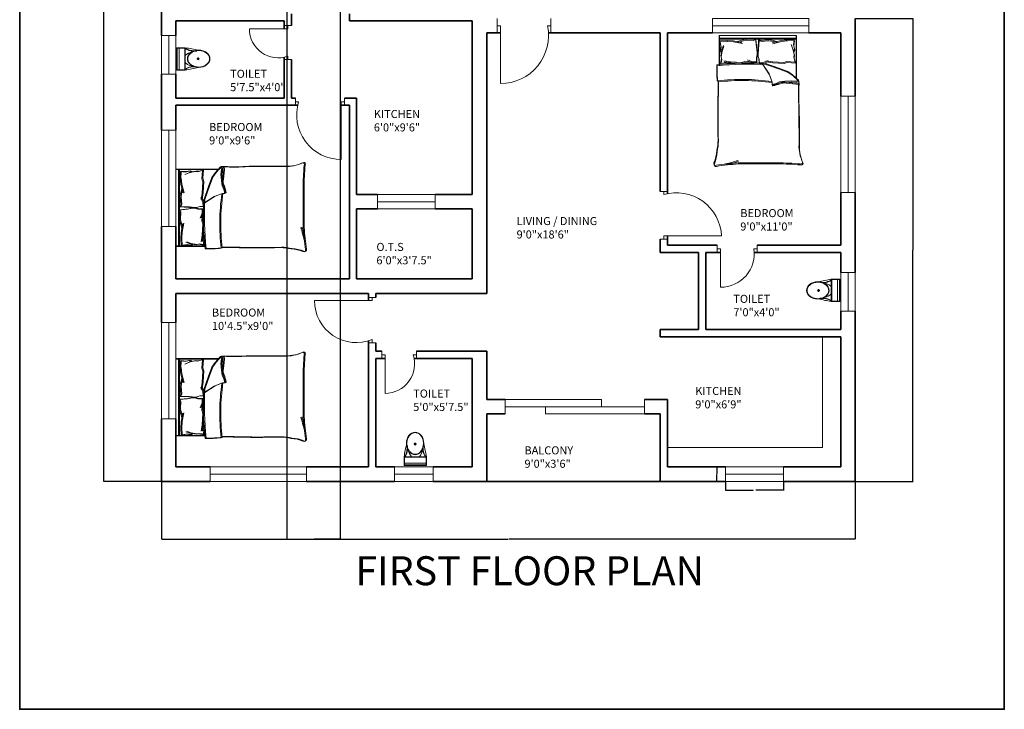
# Model space of a CAD drawing. Units: inches. Extents: x 2527 to 3140, y 1564 to 2435.
# Tile 1 of 4: x 2527 to 3140, y 1564 to 1993. Entities that reach past the tile are written whole.
import ezdxf

# ---------------------------------------------------------------- set-up
doc = ezdxf.new("R2010")
doc.units = ezdxf.units.IN
for name, color, linetype, lineweight in [('A-ANNO-DIMS', 2, 'Continuous', 18), ('A-ANNO-TEXT', 7, 'Continuous', 25), ('A-ANNO-TTLB', 7, 'Continuous', 35), ('A-AREA-IDEN', 7, 'Continuous', 18), ('A-DOOR', 191, 'Continuous', 18), ('A-FLOR-CASE', 9, 'Continuous', 18), ('A-FLOR-FIXT', 7, 'Continuous', 18), ('A-FURN', 8, 'Continuous', 13), ('A-GLAZ', 131, 'Continuous', 18), ('A-WALL', 7, 'Continuous', 35)]:
    doc.layers.add(name, color=color, linetype=linetype, lineweight=lineweight)
doc.styles.get("Standard").update_dxf_attribs({"font": 'arial.ttf'})
doc.dimstyles.get("Standard").update_dxf_attribs({"dimtxt": 0.18, "dimasz": 0.18, "dimexe": 0.18, "dimexo": 0.0625, "dimgap": 0.09, "dimtad": 0, "dimtih": 1, "dimtoh": 1, "dimdec": 4, "dimzin": 0, "dimdsep": 46, "dimtxsty": 'Standard', "dimcen": 0.09, "dimadec": 0, "dimazin": 0, "dimtfac": 1, "dimtdec": 4, "dimtofl": 0, "dimtmove": 0, "dimatfit": 3, "dimfxl": 1, "dimtolj": 1, "dimtzin": 0, "dimarcsym": 0})

# ---------------------------------------------------------------- blocks, each defined once
blk = doc.blocks.new('A$C31115884')
for p, q in [((283, 498), (223, 498)), ((258, 466), (258, 523)), ((0, 200), (0, 0)), ((520, 200), (0, 200)), ((510, 54), (0, 54)), ((10, 190), (10, 10)), ((510, 190), (10, 190)), ((10, 10), (510, 10)), ((510, 10), (510, 190)), ((520, 0), (520, 200)), ((0, 0), (520, 0))]:
    blk.add_line(p, q)
blk.add_circle((256, 496), 23.6)
for centre, radius, start, end in [((2778, -205), 2807, 165.4549, 171.7133), ((-295, 403), 365, 324.2091, 9.3499), ((-295, 403), 375, 324.2091, 9.3499), ((806, 403), 365, 170.6501, 215.7909), ((3237, 905), 2807, 188.2867, 194.5451), ((384, 406), 293, 190.2774, 224.1564), ((139, 406), 293, 315.8436, 2.6563), ((806, 403), 375, 179.2036, 215.7909)]:
    blk.add_arc(centre, radius, start, end)
blk.add_ellipse((256, 510), major_axis=(0, -261), ratio=0.772727)
blk.add_open_spline([(256, 259), (263, 259), (270, 260), (288, 262), (299, 265), (320, 273), (330, 278), (350, 291), (360, 299), (378, 316), (386, 326), (402, 347), (409, 358), (421, 383), (427, 395), (436, 422), (440, 436), (445, 465), (447, 480), (448, 509), (448, 524), (445, 553), (443, 568), (436, 596), (432, 610), (422, 636), (416, 649), (402, 672), (395, 683), (379, 703), (370, 712), (351, 728), (341, 735), (321, 746), (310, 751), (289, 757), (278, 759), (256, 761), (245, 761), (223, 757), (212, 754), (191, 746), (181, 741), (161, 728), (151, 720), (133, 703), (125, 693), (110, 672), (103, 660), (90, 636), (85, 623), (76, 596), (72, 582), (67, 553), (66, 538), (64, 509), (65, 494), (68, 465), (70, 450), (77, 422), (81, 408), (91, 382), (97, 370), (111, 346), (118, 335), (135, 316), (144, 307), (162, 291), (172, 284), (193, 273), (203, 269), (225, 262), (236, 260), (250, 259), (253, 259), (256, 259)], degree=3, knots=[0, 0, 0, 0, 0.110105, 0.110105, 0.285049, 0.285049, 0.459994, 0.459994, 0.634938, 0.634938, 0.809882, 0.809882, 0.984827, 0.984827, 1.159771, 1.159771, 1.334715, 1.334715, 1.50966, 1.50966, 1.684604, 1.684604, 1.859549, 1.859549, 2.034493, 2.034493, 2.209437, 2.209437, 2.384382, 2.384382, 2.559326, 2.559326, 2.73427, 2.73427, 2.909215, 2.909215, 3.084159, 3.084159, 3.259103, 3.259103, 3.434048, 3.434048, 3.608992, 3.608992, 3.783936, 3.783936, 3.958881, 3.958881, 4.133825, 4.133825, 4.30877, 4.30877, 4.483714, 4.483714, 4.658658, 4.658658, 4.833603, 4.833603, 5.008547, 5.008547, 5.183491, 5.183491, 5.358436, 5.358436, 5.53338, 5.53338, 5.708324, 5.708324, 5.883269, 5.883269, 6.058213, 6.058213, 6.233158, 6.233158, 6.283185, 6.283185, 6.283185, 6.283185])
blk = doc.blocks.new('BED-DOUBLE')
for p, q in [((3.48, 63.33), (3.48, 81.44)), ((3.48, 63.33), (3.48, 81.44)), ((3.48, 81.44), (51.49, 81.44)), ((3.48, 79.91), (51.27, 79.91)), ((3.48, 79.91), (51.27, 79.91)), ((3.7, 62.69), (3.7, 80.8)), ((3.7, 62.69), (3.7, 80.8)), ((51.27, 81.44), (51.27, 54.83)), ((51.27, 81.44), (51.27, 54.83)), ((51.49, 81.44), (51.49, 80.8)), ((51.49, 80.8), (51.49, 54.19)), ((51.49, 80.8), (51.49, 54.19)), ((3.7, 79.27), (51.49, 79.27)), ((3.7, 79.27), (51.49, 79.27)), ((3.89, 78.13), (4.47, 74.95)), ((3.9, 78.1), (8.18, 78.43)), ((3.9, 78.1), (8.18, 78.43)), ((3.9, 78.13), (4.47, 74.95)), ((4.47, 74.95), (4.04, 72.34)), ((4.47, 74.95), (4.04, 72.34)), ((4.12, 77.49), (4.7, 74.31)), ((4.12, 77.49), (4.7, 74.31)), ((4.13, 77.47), (8.41, 77.79)), ((4.13, 77.47), (8.41, 77.79)), ((4.7, 74.31), (4.27, 71.7)), ((4.7, 74.31), (4.27, 71.7)), ((5.05, 72.49), (6.06, 75.24)), ((5.05, 72.49), (6.06, 75.24)), ((5.28, 71.85), (6.29, 74.6)), ((5.28, 71.85), (6.29, 74.6)), ((8.18, 78.43), (8.29, 78.42)), ((8.18, 78.43), (8.29, 78.42)), ((8.29, 78.42), (12.11, 78.13)), ((8.29, 78.42), (12.11, 78.13)), ((8.41, 77.79), (8.51, 77.78)), ((8.41, 77.79), (8.51, 77.78)), ((8.51, 77.78), (12.34, 77.49)), ((8.51, 77.78), (12.34, 77.49)), ((12.11, 78.13), (17.6, 77.11)), ((12.11, 78.13), (17.6, 77.11)), ((12.34, 77.49), (17.83, 76.48)), ((12.34, 77.49), (17.83, 76.48)), ((14.86, 77.69), (16.88, 78.42)), ((14.86, 77.69), (16.88, 78.42)), ((15.08, 77.05), (17.11, 77.78)), ((15.08, 77.05), (17.11, 77.78)), ((16.88, 78.42), (19.77, 79.14)), ((16.88, 78.42), (19.77, 79.14)), ((17.11, 77.78), (20, 78.5)), ((17.11, 77.78), (20, 78.5)), ((19.77, 79.14), (20.09, 79.14)), ((19.77, 79.14), (20.09, 79.14)), ((20, 78.5), (20.32, 78.5)), ((20, 78.5), (20.32, 78.5)), ((20.09, 79.14), (24.54, 78.99)), ((20.09, 79.14), (24.54, 78.99)), ((20.32, 78.5), (24.77, 78.35)), ((20.32, 78.5), (24.77, 78.35)), ((24.54, 78.99), (25.98, 79.57)), ((24.54, 78.99), (25.98, 79.57)), ((24.77, 78.35), (26.21, 78.93)), ((24.77, 78.35), (26.21, 78.93)), ((25.98, 79.57), (26.56, 74.22)), ((25.98, 79.57), (26.56, 74.22)), ((26.21, 78.93), (26.79, 73.58)), ((26.21, 78.93), (26.79, 73.58)), ((26.56, 74.22), (27.14, 71.04)), ((26.56, 74.22), (27.14, 71.04)), ((26.79, 73.58), (27.37, 70.4)), ((26.79, 73.58), (27.37, 70.4)), ((27.73, 73.58), (27.36, 70.36)), ((27.73, 73.58), (27.36, 70.36)), ((27.98, 78.95), (27.73, 73.58)), ((27.98, 78.95), (27.73, 73.58)), ((28.21, 78.31), (27.96, 72.94)), ((28.21, 78.31), (27.96, 72.94)), ((29.46, 78.46), (27.98, 78.95)), ((29.46, 78.46), (27.98, 78.95)), ((29.68, 77.82), (28.21, 78.31)), ((29.68, 77.82), (28.21, 78.31)), ((33.88, 78.89), (29.46, 78.46)), ((33.88, 78.89), (29.46, 78.46)), ((34.11, 78.25), (29.68, 77.82)), ((34.11, 78.25), (29.68, 77.82)), ((34.21, 78.91), (33.88, 78.89)), ((34.2, 78.91), (33.88, 78.89)), ((34.43, 78.27), (34.11, 78.25)), ((34.43, 78.27), (34.11, 78.25)), ((37.14, 78.36), (34.2, 78.91)), ((37.14, 78.36), (34.21, 78.91)), ((37.36, 77.73), (34.43, 78.27)), ((37.36, 77.73), (34.43, 78.27)), ((41.91, 78.37), (36.5, 77.02)), ((41.91, 78.37), (36.5, 77.02)), ((42.14, 77.73), (36.72, 76.38)), ((42.14, 77.73), (36.72, 76.38)), ((39.2, 77.77), (37.14, 78.36)), ((39.2, 77.77), (37.14, 78.36)), ((39.43, 77.13), (37.36, 77.73)), ((39.43, 77.13), (37.36, 77.73)), ((45.71, 78.9), (41.91, 78.37)), ((45.71, 78.9), (41.91, 78.37)), ((45.94, 78.26), (42.14, 77.73)), ((45.94, 78.26), (42.14, 77.73)), ((50.11, 78.89), (44.71, 78.98)), ((44.71, 78.98), (45.71, 78.9)), ((50.11, 78.89), (44.71, 78.98)), ((44.71, 78.98), (45.71, 78.9)), ((50.34, 78.25), (44.94, 78.34)), ((44.94, 78.34), (45.94, 78.26)), ((50.34, 78.25), (44.94, 78.34)), ((44.94, 78.34), (45.94, 78.26)), ((49.31, 73.19), (48.13, 75.86)), ((49.31, 73.19), (48.13, 75.86)), ((49.54, 72.55), (48.36, 75.23)), ((49.54, 72.55), (48.36, 75.23)), ((50.11, 78.89), (49.73, 75.68)), ((50.11, 78.89), (49.73, 75.68)), ((49.73, 75.68), (50.33, 73.1)), ((49.73, 75.68), (50.33, 73.1)), ((50.34, 78.25), (49.96, 75.04)), ((50.34, 78.25), (49.96, 75.04)), ((49.96, 75.04), (50.56, 72.47)), ((49.96, 75.04), (50.56, 72.47)), ((4.04, 72.34), (4.62, 71.33)), ((4.04, 72.34), (4.62, 71.33)), ((4.27, 71.7), (4.85, 70.69)), ((4.27, 71.7), (4.85, 70.69)), ((4.47, 68.87), (5.05, 72.49)), ((4.47, 68.87), (5.05, 72.49)), ((4.76, 67.28), (4.47, 68.87)), ((4.76, 67.28), (4.47, 68.87)), ((4.7, 68.23), (5.28, 71.85)), ((4.7, 68.23), (5.28, 71.85)), ((4.99, 66.64), (4.7, 68.23)), ((4.99, 66.64), (4.7, 68.23)), ((27.14, 69.74), (26.56, 67.86)), ((27.14, 69.74), (26.56, 67.86)), ((26.56, 67.86), (26.56, 65.18)), ((26.56, 67.86), (26.56, 65.18)), ((27.37, 69.1), (26.79, 67.22)), ((27.37, 69.1), (26.79, 67.22)), ((27.14, 71.04), (27.14, 69.74)), ((27.14, 71.04), (27.14, 69.74)), ((27.36, 70.36), (27.44, 69.07)), ((27.36, 70.36), (27.44, 69.07)), ((27.37, 70.4), (27.37, 69.1)), ((27.37, 70.4), (27.37, 69.1)), ((27.44, 69.07), (28.13, 67.23)), ((27.44, 69.07), (28.13, 67.23)), ((27.96, 72.94), (27.58, 69.73)), ((27.96, 72.94), (27.58, 69.73)), ((27.58, 69.73), (27.66, 68.43)), ((27.58, 69.73), (27.66, 68.43)), ((27.66, 68.43), (28.36, 66.59)), ((27.66, 68.43), (28.36, 66.59)), ((50.11, 69.61), (49.31, 73.19)), ((50.11, 69.61), (49.31, 73.19)), ((50.34, 68.97), (49.54, 72.55)), ((50.34, 68.97), (49.54, 72.55)), ((50.33, 73.1), (49.81, 72.06)), ((50.33, 73.1), (49.82, 72.06)), ((49.92, 68.01), (50.11, 69.61)), ((49.92, 68.01), (50.11, 69.61)), ((50.7, 64.87), (49.92, 68.01)), ((50.7, 64.87), (49.92, 68.01)), ((50.56, 72.47), (50.04, 71.42)), ((50.56, 72.47), (50.04, 71.42)), ((50.15, 67.37), (50.34, 68.97)), ((50.15, 67.37), (50.34, 68.97)), ((4.18, 64.1), (4.76, 67.28)), ((4.18, 64.1), (4.76, 67.28)), ((9.28, 64.82), (4.18, 64.1)), ((9.28, 64.82), (4.18, 64.1)), ((4.41, 63.46), (4.99, 66.64)), ((4.41, 63.46), (4.99, 66.64)), ((9.51, 64.19), (4.41, 63.46)), ((9.51, 64.19), (4.41, 63.46)), ((6.38, 65.81), (10.41, 65.15)), ((6.38, 65.81), (10.41, 65.15)), ((6.61, 65.17), (10.64, 64.51)), ((6.61, 65.17), (10.64, 64.51)), ((10.41, 65.15), (9.28, 64.82)), ((10.41, 65.15), (9.28, 64.82)), ((10.64, 64.51), (9.51, 64.19)), ((10.64, 64.51), (9.51, 64.19)), ((10.41, 65.15), (17.42, 64.72)), ((10.41, 65.15), (17.42, 64.72)), ((10.64, 64.51), (17.65, 64.08)), ((10.64, 64.51), (17.65, 64.08)), ((17.42, 64.72), (19.38, 65.27)), ((17.42, 64.72), (19.38, 65.27)), ((17.65, 64.08), (19.61, 64.63)), ((17.65, 64.08), (19.61, 64.63)), ((19.38, 65.27), (24.52, 64.87)), ((19.38, 65.27), (24.52, 64.87)), ((19.61, 64.63), (24.74, 64.23)), ((19.61, 64.63), (24.74, 64.23)), ((24.1, 65.18), (20.96, 66.27)), ((24.1, 65.18), (20.96, 66.27)), ((24.33, 64.54), (21.19, 65.63)), ((24.33, 64.54), (21.19, 65.63)), ((26.56, 65.18), (24.1, 65.18)), ((26.56, 65.18), (24.1, 65.18)), ((26.79, 64.54), (24.33, 64.54)), ((26.79, 64.54), (24.33, 64.54)), ((26.79, 67.22), (26.79, 64.54)), ((26.79, 67.22), (26.79, 64.54)), ((28.13, 67.23), (28.3, 64.55)), ((28.13, 67.23), (28.3, 64.55)), ((28.3, 64.55), (30.75, 64.7)), ((28.3, 64.55), (30.75, 64.7)), ((28.36, 66.59), (28.53, 63.91)), ((28.36, 66.59), (28.53, 63.91)), ((28.53, 63.91), (30.98, 64.06)), ((28.53, 63.91), (30.98, 64.06)), ((30.26, 64.06), (34.45, 57.57)), ((30.26, 64.06), (34.45, 57.57)), ((30.49, 63.42), (34.68, 56.93)), ((30.49, 63.42), (34.68, 56.93)), ((30.75, 64.7), (33.82, 65.99)), ((30.75, 64.7), (33.82, 65.99)), ((30.98, 64.06), (34.05, 65.35)), ((30.98, 64.06), (34.05, 65.35)), ((40.64, 61.13), (32.31, 64.06)), ((40.64, 61.13), (32.31, 64.06)), ((40.87, 60.49), (32.53, 63.42)), ((40.87, 60.49), (32.54, 63.42)), ((32.56, 65.81), (36.6, 65.15)), ((32.56, 65.81), (36.6, 65.15)), ((32.79, 65.17), (36.83, 64.51)), ((32.79, 65.17), (36.82, 64.51)), ((36.6, 65.15), (43.61, 64.72)), ((36.6, 65.15), (43.61, 64.72)), ((36.82, 64.51), (43.83, 64.08)), ((36.83, 64.51), (43.84, 64.08)), ((43.61, 64.72), (45.57, 65.27)), ((43.61, 64.72), (45.57, 65.27)), ((43.83, 64.08), (45.8, 64.63)), ((43.84, 64.08), (45.8, 64.63)), ((45.57, 65.27), (50.7, 64.87)), ((45.57, 65.27), (50.7, 64.87)), ((45.8, 64.63), (50.93, 64.23)), ((45.8, 64.63), (50.93, 64.23)), ((50.93, 64.23), (50.15, 67.37)), ((50.93, 64.23), (50.15, 67.37)), ((34.45, 57.57), (36.15, 53.08)), ((34.45, 57.57), (36.15, 53.08)), ((34.68, 56.93), (36.38, 52.44)), ((34.68, 56.93), (36.38, 52.44)), ((46.22, 59.11), (40.64, 61.13)), ((46.22, 59.11), (40.64, 61.13)), ((46.45, 58.47), (40.87, 60.49)), ((46.45, 58.47), (40.87, 60.49)), ((49.16, 56.95), (46.22, 59.11)), ((49.16, 56.95), (46.22, 59.11)), ((49.39, 56.31), (46.45, 58.47)), ((49.39, 56.31), (46.45, 58.47)), ((52.87, 53.7), (49.16, 56.95)), ((52.87, 53.7), (49.16, 56.95)), ((53.1, 53.06), (49.39, 56.31)), ((53.1, 53.06), (49.39, 56.31)), ((36.15, 53.08), (36.46, 51.07)), ((36.15, 53.08), (36.46, 51.07)), ((36.38, 52.44), (36.69, 50.43)), ((36.38, 52.44), (36.69, 50.43)), ((36.46, 51.07), (38.94, 51.68)), ((36.46, 51.07), (38.94, 51.68)), ((36.69, 50.43), (39.17, 51.05)), ((36.69, 50.43), (39.17, 51.05)), ((38.94, 51.68), (40.95, 52.61)), ((38.94, 51.68), (40.95, 52.61)), ((39.17, 51.05), (41.18, 51.97)), ((39.17, 51.05), (41.18, 51.97)), ((40.95, 52.61), (44.36, 53.08)), ((40.95, 52.61), (44.36, 53.08)), ((41.18, 51.97), (44.59, 52.44)), ((41.18, 51.97), (44.59, 52.44)), ((44.36, 53.08), (48.23, 53.39)), ((44.36, 53.08), (48.23, 53.39)), ((44.59, 52.44), (48.46, 52.75)), ((44.59, 52.44), (48.46, 52.75)), ((48.23, 53.39), (51.33, 53.08)), ((48.23, 53.39), (51.33, 53.08)), ((48.46, 52.75), (51.56, 52.44)), ((48.46, 52.75), (51.56, 52.44)), ((51.33, 53.08), (52.87, 53.7)), ((51.33, 53.08), (52.87, 53.7)), ((51.56, 52.44), (53.1, 53.06)), ((51.56, 52.44), (53.1, 53.06)), ((52.95, 51.95), (52.87, 53.7, 3.87)), ((52.95, 51.95), (52.87, 53.7, 3.87)), ((53.18, 51.31), (53.1, 53.06, 3.87)), ((53.18, 51.31), (53.1, 53.06, 3.87)), ((15.06, 2.2), (39.68, 2.2)), ((15.06, 2.2), (39.68, 2.2)), ((15.29, 1.56), (39.91, 1.56)), ((15.29, 1.56), (39.91, 1.56))]:
    blk.add_line(p, q)
for centre, radius, start, end in [((85.16, 61.35), 83.31, 178.72178, 185.60397), ((85.16, 61.35), 83.31, 178.72178, 185.60397), ((21.36, -100.61), 164.97, 86.08655, 96.78213), ((21.36, -100.61), 164.97, 86.08655, 96.78213), ((85.39, 60.71), 83.31, 178.72178, 185.60397), ((85.39, 60.71), 83.31, 178.72178, 185.60397), ((21.59, -101.25), 164.97, 86.08655, 96.78213), ((21.59, -101.25), 164.97, 86.08655, 96.78213), ((17.76, -74.87), 129.02, 81.78449, 96.90062), ((17.76, -74.87), 129.02, 81.78449, 96.90062), ((17.98, -75.51), 129.02, 81.78449, 96.90062), ((17.98, -75.51), 129.02, 81.78449, 96.90062), ((-167.31, 50.27), 170.11, 358.4762, 1.00819), ((-167.31, 50.27), 170.11, 358.4762, 1.00819), ((-167.08, 49.63), 170.11, 358.4762, 1.00819), ((-167.08, 49.63), 170.11, 358.4762, 1.00819), ((36.64, 51), 0.185, 160.24637, 271.13765), ((36.64, 51), 0.185, 160.24637, 271.13765), ((31.15, 79.96), 29.65, 280.66171, 289.88058), ((31.15, 79.96), 29.65, 280.66171, 289.88058), ((36.87, 50.36), 0.185, 160.24637, 271.13765), ((36.86, 50.36), 0.185, 160.24637, 271.13765), ((31.38, 79.32), 29.65, 280.66171, 289.88058), ((31.38, 79.32), 29.65, 280.66171, 289.88058), ((43.74, 46.38), 6.22, 78.6608, 113.73842), ((43.74, 46.38), 6.22, 78.6608, 113.73842), ((43.97, 45.74), 6.22, 78.6608, 113.73842), ((43.97, 45.74), 6.22, 78.6608, 113.73842), ((51.33, 88.1), 36.18, 259.87628, 272.56571), ((51.33, 88.1), 36.18, 259.87628, 272.56571), ((51.56, 87.46), 36.18, 259.87628, 272.56571), ((51.56, 87.46), 36.18, 259.87628, 272.56571), ((182.27, 45.13), 129.5, 176.97912, 183.83645), ((182.27, 45.13), 129.5, 176.97912, 183.83645), ((182.49, 44.49), 129.5, 176.97912, 183.83645), ((182.49, 44.49), 129.5, 176.97912, 183.83645), ((484.82, 30.83), 482.31, 178.22771, 181.71854), ((484.82, 30.83), 482.31, 178.22771, 181.71854), ((485.05, 30.19), 482.31, 178.22771, 181.71854), ((485.05, 30.19), 482.31, 178.22771, 181.71854), ((-4508.74, 13.62), 4561.86, 0.00217, 0.28689), ((-4508.74, 13.62), 4561.86, 0.00217, 0.28689), ((-4508.51, 12.98), 4561.86, 0.00217, 0.28689), ((-4508.51, 12.98), 4561.86, 0.00217, 0.28689), ((-26.9, 16.93), 29.63, 346.06484, 358.91125), ((-26.9, 16.93), 29.63, 346.06484, 358.91125), ((-26.67, 16.29), 29.63, 346.06484, 358.91125), ((-26.67, 16.29), 29.63, 346.06484, 358.91125), ((76.16, 12.78), 23.07, 177.47136, 206.46809), ((76.16, 12.78), 23.07, 177.47136, 206.46809), ((76.39, 12.14), 23.07, 177.47136, 206.46809), ((76.39, 12.14), 23.07, 177.47136, 206.46809), ((-21.66, 11.17), 23.56, 337.97508, 356.652), ((-21.66, 11.17), 23.56, 337.97508, 356.652), ((-21.43, 10.53), 23.56, 337.97508, 356.652), ((-21.43, 10.53), 23.56, 337.97508, 356.652), ((1.09, 1.73), 1.09, 146.17358, 293.47814), ((1.09, 1.73), 1.09, 146.17358, 293.47814), ((1.32, 1.09), 1.09, 146.17358, 293.47814), ((1.32, 1.09), 1.09, 146.17358, 293.47814), ((21.43, -119.39), 121.76, 92.99578, 99.40907), ((21.43, -119.39), 121.76, 92.99578, 99.40907), ((21.66, -120.03), 121.76, 92.99578, 99.40907), ((21.66, -120.03), 121.76, 92.99578, 99.40907), ((-17.22, 105.15), 106.46, 283.38322, 287.70533), ((-17.22, 105.15), 106.46, 283.38322, 287.70533), ((-16.99, 104.52), 106.46, 283.38322, 287.70533), ((-16.99, 104.52), 106.46, 283.38322, 287.70533), ((41.15, -130.83), 133.04, 84.4998, 90.63509), ((41.15, -130.83), 133.04, 84.4998, 90.63509), ((41.38, -131.47), 133.04, 84.4998, 90.63509), ((41.38, -131.47), 133.04, 84.4998, 90.63509), ((54.41, 2.57), 1.1, 242.65876, 356.02002), ((54.41, 2.57), 1.1, 242.65876, 356.02002), ((54.64, 1.93), 1.1, 242.65876, 356.02002), ((54.64, 1.93), 1.1, 242.65876, 356.02002)]:
    blk.add_arc(centre, radius, start, end)
blk = doc.blocks.new('WIN-60')
for p, q in [((0, 9), (0, 0)), ((60, 9), (0, 9)), ((60, 4.5), (60, 9)), ((60, 9), (60, 0)), ((0, 0), (0, 4.5)), ((0, 4.5), (60, 4.5)), ((0, 0), (60, 0))]:
    blk.add_line(p, q)
blk = doc.blocks.new('WIN-24')
for p, q in [((4.5, 24), (0, 24)), ((0, 24), (9, 24)), ((0, 24), (0, 0)), ((4.5, 0), (4.5, 24)), ((9, 24), (9, 0)), ((0, 0), (9, 0)), ((9, 0), (4.5, 0))]:
    blk.add_line(p, q)
blk = doc.blocks.new('WIN-36')
for p, q in [((0, 36), (9, 36)), ((0, 36), (0, 0)), ((9, 36), (4.5, 36)), ((4.5, 36), (4.5, 0)), ((9, 36), (9, 0)), ((4.5, 0), (0, 0)), ((0, 0), (9, 0))]:
    blk.add_line(p, q)
blk = doc.blocks.new('*D15')
at = {"layer": 'A-ANNO-DIMS', "color": 0, "lineweight": -2, "transparency": 16777216}
for p, q in [((2966.88, 1706.08), (2966.88, 1700.56)), ((3002.88, 1706.08), (3002.88, 1700.56)), ((2967.06, 1700.74), (2984.03, 1700.74)), ((3002.7, 1700.74), (2985.72, 1700.74))]:
    blk.add_line(p, q, dxfattribs=at)
at = {"layer": 'A-ANNO-DIMS', "color": 0, "transparency": 16777216}
for points in [[(2967.06, 1700.77), (2967.06, 1700.71), (2966.88, 1700.74)], [(3002.7, 1700.77), (3002.7, 1700.71), (3002.88, 1700.74)]]:
    blk.add_solid(points, dxfattribs=at)
at = {"layer": 'Defpoints', "color": 0, "transparency": 16777216}
for p in [(2966.88, 1706.14), (3002.88, 1706.14), (2966.88, 1700.74)]:
    blk.add_point(p, dxfattribs=at)
at = {"layer": 'A-ANNO-DIMS', "color": 0, "transparency": 16777216, "insert": (2984.88, 1700.74), "char_height": 0.18, "attachment_point": 5}
blk.add_mtext('\\A1;WIN. 36 TYP.', dxfattribs=at)
blk = doc.blocks.new('*D16')
at = {"layer": 'A-ANNO-DIMS', "color": 0, "lineweight": -2, "transparency": 16777216}
for p, q in [((2966.82, 1715.14), (2961.3, 1715.14)), ((2961.48, 1714.96), (2961.48, 1710.82)), ((2966.82, 1706.14), (2961.3, 1706.14)), ((2961.48, 1706.32), (2961.48, 1710.46))]:
    blk.add_line(p, q, dxfattribs=at)
at = {"layer": 'A-ANNO-DIMS', "color": 0, "transparency": 16777216}
for points in [[(2961.45, 1714.96), (2961.51, 1714.96), (2961.48, 1715.14)], [(2961.45, 1706.32), (2961.51, 1706.32), (2961.48, 1706.14)]]:
    blk.add_solid(points, dxfattribs=at)
at = {"layer": 'Defpoints', "color": 0, "transparency": 16777216}
for p in [(2961.48, 1715.14), (2966.88, 1715.14), (2966.88, 1706.14)]:
    blk.add_point(p, dxfattribs=at)
at = {"layer": 'A-ANNO-DIMS', "color": 0, "transparency": 16777216, "insert": (2961.48, 1710.64), "char_height": 0.18, "attachment_point": 5}
blk.add_mtext('\\A1;9 TYP.', dxfattribs=at)
blk = doc.blocks.new('*D19')
at = {"layer": 'A-ANNO-DIMS', "color": 0, "lineweight": -2, "transparency": 16777216}
for p, q in [((2615.58, 1706.08), (2615.58, 1670.11)), ((3047.58, 1706.08), (3047.58, 1670.11)), ((2615.76, 1670.29), (2831.29, 1670.29)), ((3047.4, 1670.29), (2831.87, 1670.29))]:
    blk.add_line(p, q, dxfattribs=at)
at = {"layer": 'A-ANNO-DIMS', "color": 0, "transparency": 16777216}
for points in [[(2615.76, 1670.32), (2615.76, 1670.26), (2615.58, 1670.29)], [(3047.4, 1670.32), (3047.4, 1670.26), (3047.58, 1670.29)]]:
    blk.add_solid(points, dxfattribs=at)
at = {"layer": 'Defpoints', "color": 0, "transparency": 16777216}
for p in [(2615.58, 1706.14), (3047.58, 1706.14), (3047.58, 1670.29)]:
    blk.add_point(p, dxfattribs=at)
at = {"layer": 'A-ANNO-DIMS', "color": 0, "transparency": 16777216, "insert": (2831.58, 1670.29), "char_height": 0.18, "attachment_point": 5}
blk.add_mtext('\\A1;432', dxfattribs=at)
blk = doc.blocks.new('*D20')
at = {"layer": 'A-ANNO-DIMS', "color": 0, "lineweight": -2, "transparency": 16777216}
for p, q in [((2615.52, 2348.14), (2579.55, 2348.14)), ((2579.73, 2347.96), (2579.73, 2027.32)), ((2579.73, 1706.32), (2579.73, 2026.96)), ((2615.52, 1706.14), (2579.55, 1706.14))]:
    blk.add_line(p, q, dxfattribs=at)
at = {"layer": 'A-ANNO-DIMS', "color": 0, "transparency": 16777216}
for points in [[(2579.7, 2347.96), (2579.76, 2347.96), (2579.73, 2348.14)], [(2579.7, 1706.32), (2579.76, 1706.32), (2579.73, 1706.14)]]:
    blk.add_solid(points, dxfattribs=at)
at = {"layer": 'Defpoints', "color": 0, "transparency": 16777216}
for p in [(2579.73, 2348.14), (2615.58, 2348.14), (2615.58, 1706.14)]:
    blk.add_point(p, dxfattribs=at)
at = {"layer": 'A-ANNO-DIMS', "color": 0, "transparency": 16777216, "insert": (2579.73, 2027.14), "char_height": 0.18, "attachment_point": 5}
blk.add_mtext('\\A1;642', dxfattribs=at)
blk = doc.blocks.new('*D23')
at = {"layer": 'A-ANNO-DIMS', "color": 0, "lineweight": -2, "transparency": 16777216}
for p, q in [((3047.64, 1994.14), (3083.61, 1994.14)), ((3083.43, 1993.96), (3083.43, 1850.32)), ((3083.43, 1706.32), (3083.43, 1849.96)), ((3047.64, 1706.14), (3083.61, 1706.14))]:
    blk.add_line(p, q, dxfattribs=at)
at = {"layer": 'A-ANNO-DIMS', "color": 0, "transparency": 16777216}
for points in [[(3083.4, 1993.96), (3083.46, 1993.96), (3083.43, 1994.14)], [(3083.4, 1706.32), (3083.46, 1706.32), (3083.43, 1706.14)]]:
    blk.add_solid(points, dxfattribs=at)
at = {"layer": 'Defpoints', "color": 0, "transparency": 16777216}
for p in [(3047.58, 1994.14), (3083.43, 1994.14), (3047.58, 1706.14)]:
    blk.add_point(p, dxfattribs=at)
at = {"layer": 'A-ANNO-DIMS', "color": 0, "transparency": 16777216, "insert": (3083.43, 1850.14), "char_height": 0.18, "attachment_point": 5}
blk.add_mtext('\\A1;288', dxfattribs=at)
blk = doc.blocks.new('*D33')
at = {"layer": 'A-ANNO-DIMS', "color": 0, "lineweight": -2, "transparency": 16777216}
for p, q in [((2693.66, 2105.08), (2693.66, 1670.11)), ((2726.85, 2105.08), (2726.85, 1670.11)), ((2693.84, 1670.29), (2709.86, 1670.29)), ((2726.67, 1670.29), (2710.65, 1670.29))]:
    blk.add_line(p, q, dxfattribs=at)
at = {"layer": 'A-ANNO-DIMS', "color": 0, "transparency": 16777216}
for points in [[(2693.84, 1670.32), (2693.84, 1670.26), (2693.66, 1670.29)], [(2726.67, 1670.32), (2726.67, 1670.26), (2726.85, 1670.29)]]:
    blk.add_solid(points, dxfattribs=at)
at = {"layer": 'Defpoints', "color": 0, "transparency": 16777216}
for p in [(2693.66, 2105.14), (2726.85, 2105.14), (2726.85, 1670.29)]:
    blk.add_point(p, dxfattribs=at)
at = {"layer": 'A-ANNO-DIMS', "color": 0, "transparency": 16777216, "insert": (2710.25, 1670.29), "char_height": 0.18, "attachment_point": 5}
blk.add_mtext('\\A1;33.18', dxfattribs=at)

msp = doc.modelspace()

# ---------------------------------------------------------------- linework, layer by layer
at = {"layer": 'A-ANNO-TTLB'}
msp.add_lwpolyline([(2527.301, 2435.1781), (3140.3962, 2435.1781), (3140.3962, 1564.3652), (2527.301, 1564.3652)], close=True, dxfattribs=at)
at = {"layer": 'A-DOOR'}
for p, q in [((2824.6085, 1994.1426), (2824.6085, 1985.1426)), ((2857.9902, 1994.1426), (2857.9902, 1985.1426)), ((2694.3292, 1987.7114), (2670.3292, 1987.7114)), ((2692.0792, 1989.7114), (2696.5792, 1989.7114)), ((2696.5792, 1989.7114), (2694.3292, 1989.7114)), ((2694.3292, 1989.7114), (2694.3292, 1987.7114)), ((2824.6085, 1985.1426), (2824.6085, 1989.6426)), ((2824.6085, 1989.6426), (2826.6085, 1989.6426)), ((2826.6085, 1989.6426), (2826.6085, 1953.6426)), ((2857.9902, 1989.6426), (2855.9902, 1989.6426)), ((2857.9902, 1985.1426), (2857.9902, 1989.6426)), ((2692.0792, 1968.6426), (2696.5792, 1968.6426)), ((2694.3292, 1968.6426), (2694.3292, 1970.6426)), ((2696.5792, 1968.6426), (2694.3292, 1968.6426)), ((2698.9779, 1944.6426), (2698.9779, 1940.1426)), ((2729.551, 1940.1426), (2729.551, 1944.6426)), ((2729.551, 1944.6426), (2729.551, 1942.3926)), ((2698.9779, 1940.1426), (2698.9779, 1942.3926)), ((2698.9779, 1942.3926), (2700.9779, 1942.3926)), ((2729.551, 1942.3926), (2727.551, 1942.3926)), ((2727.551, 1942.3926), (2727.551, 1906.3926)), ((2926.0792, 1886.5901), (2930.5792, 1886.5901)), ((2930.5792, 1886.5901), (2928.3292, 1886.5901)), ((2928.3292, 1886.5901), (2928.3292, 1884.5901)), ((2928.3292, 1856.8415), (2928.3292, 1858.8415)), ((2928.3292, 1858.8415), (2964.3292, 1858.8415)), ((2926.0792, 1856.8415), (2930.5792, 1856.8415)), ((2930.5792, 1856.8415), (2928.3292, 1856.8415)), ((2928.3292, 1856.8415), (2929.4542, 1856.8415)), ((2929.4542, 1856.8415), (2928.3292, 1856.8415)), ((2961.6794, 1853.1426), (2961.6794, 1848.6426)), ((2986.5173, 1853.1426), (2986.5173, 1848.6426)), ((2961.6794, 1848.6426), (2961.6794, 1850.8926)), ((2961.6794, 1850.8926), (2963.6794, 1850.8926)), ((2963.6794, 1850.8926), (2963.6794, 1826.8926)), ((2986.5173, 1850.8926), (2984.5173, 1850.8926)), ((2986.5173, 1848.6426), (2986.5173, 1850.8926)), ((2746.8292, 1818.6245), (2710.8292, 1818.6245)), ((2744.5792, 1820.6245), (2749.0792, 1820.6245)), ((2749.0792, 1820.6245), (2746.8292, 1820.6245)), ((2746.8292, 1820.6245), (2746.8292, 1818.6245)), ((2744.5792, 1792.4277), (2749.0792, 1792.4277)), ((2746.8292, 1792.4277), (2746.8292, 1794.4277)), ((2752.8291, 1787.1426), (2752.8291, 1782.6426)), ((2752.8291, 1782.6426), (2752.8291, 1784.8926)), ((2752.8291, 1784.8926), (2754.8291, 1784.8926)), ((2754.8291, 1784.8926), (2754.8291, 1760.8926)), ((2774.3054, 1784.8926), (2772.3054, 1784.8926)), ((2774.3054, 1787.1426), (2774.3054, 1782.6426)), ((2774.3054, 1782.6426), (2774.3054, 1784.8926)), ((2829.5714, 1757.1426), (2829.5714, 1748.1426)), ((2889.6681, 1757.1426), (2829.5714, 1757.1426)), ((2889.6681, 1752.6426), (2889.6681, 1757.1426)), ((2916.276, 1752.6426), (2916.276, 1757.1426)), ((2916.276, 1757.1426), (2916.276, 1748.1426)), ((2829.5714, 1748.1426), (2829.5714, 1752.6426)), ((2829.5714, 1752.6426), (2916.276, 1752.6426)), ((2829.5714, 1748.1426), (2829.5714, 1748.1426)), ((2854.6255, 1752.6426), (2854.6255, 1748.1426)), ((2854.6255, 1748.1426), (2916.276, 1748.1426))]:
    msp.add_line(p, q, dxfattribs=at)
for centre, radius, start, end in [((2688.3989, 1987.7114), 18.0697, 180, 289.1590642), ((2826.6085, 1983.6325), 29.99, 270, 11.5603681), ((2727.551, 1934.1999), 27.8073, 162.8650473, 270), ((2936.2353, 1857.6032), 28.1212, 2.5238607, 106.3284503), ((2963.6794, 1847.9387), 21.0462, 270, 8.0681353), ((2736.9609, 1818.6245), 26.1317, 180, 292.1872601), ((2754.8291, 1779.2555), 18.3629, 270, 17.8775209)]:
    msp.add_arc(centre, radius, start, end, dxfattribs=at)
at = {"layer": 'A-FLOR-CASE'}
for p, q in [((3027.2039, 1796.1426), (3027.2039, 1727.1587)), ((3027.2039, 1727.1587), (2930.5792, 1727.1587))]:
    msp.add_line(p, q, dxfattribs=at)
at = {"layer": 'A-WALL'}
for p, q in [((2615.5792, 2022.3928), (2615.5792, 1983.547)), ((2624.5792, 1992.6426), (2624.5792, 1992.6426)), ((2624.5792, 1992.6426), (2624.5792, 1983.547)), ((2692.0792, 1992.6426), (2624.5792, 1992.6426)), ((2624.5792, 1992.6426), (2624.5792, 1983.547)), ((2692.0792, 1987.7114), (2692.0792, 1992.6426)), ((2696.5792, 1992.6426), (2696.5792, 1997.1426)), ((2696.5792, 1992.6426), (2696.5792, 1989.7114)), ((2732.5792, 1992.6426), (2732.5792, 1997.1426)), ((2809.0792, 1992.6426), (2732.5792, 1992.6426)), ((2732.5792, 1992.6426), (2737.0792, 1992.6426)), ((2809.0792, 1992.6426), (2809.0792, 1884.6426)), ((3047.5792, 1994.1426), (3047.5792, 1945.9238)), ((2818.0792, 1985.1426), (2826.6085, 1985.1426)), ((2818.0792, 1985.1426), (2818.0792, 1823.1426)), ((2856.5605, 1985.1426), (2926.0792, 1985.1426)), ((2926.0792, 1886.5901), (2926.0792, 1985.1426)), ((2930.5792, 1985.1426), (2930.5792, 1885.1497)), ((2930.5792, 1985.1426), (2958.601, 1985.1426)), ((3018.601, 1985.1426), (3038.5792, 1985.1426)), ((3038.5792, 1985.1426), (3038.5792, 1945.9238)), ((2692.0792, 1944.6426), (2692.0792, 1970.0205)), ((2696.5792, 1968.6426), (2696.5792, 1944.6426)), ((2615.5792, 1959.547), (2615.5792, 1924.7584)), ((2624.5792, 1959.547), (2624.5792, 1944.6426)), ((2624.5792, 1959.547), (2624.5792, 1944.6426)), ((2624.5792, 1944.6426), (2692.0792, 1944.6426)), ((2696.5792, 1944.6426), (2698.9779, 1944.6426)), ((2729.551, 1944.6426), (2737.0792, 1944.6426)), ((2737.0792, 1944.6426), (2737.0792, 1884.6426)), ((2696.5792, 1940.1426), (2624.5792, 1940.1426)), ((2624.5792, 1940.1426), (2624.5792, 1924.7584)), ((2696.5792, 1940.1426), (2700.3861, 1940.1426)), ((2727.551, 1940.1426), (2732.5792, 1940.1426)), ((2732.5792, 1832.1426), (2732.5792, 1940.1426)), ((2750.0181, 1884.6426), (2737.0792, 1884.6426)), ((2809.0792, 1884.6426), (2786.0181, 1884.6426)), ((3038.5792, 1885.9238), (3038.5792, 1853.1426)), ((3047.5792, 1885.9238), (3047.5792, 1836.0225)), ((2737.0792, 1832.1426), (2737.0792, 1875.6426)), ((2737.0792, 1875.6426), (2750.0181, 1875.6426)), ((2737.0792, 1875.6426), (2737.0792, 1832.1426)), ((2786.0181, 1875.6426), (2809.0792, 1875.6426)), ((2809.0792, 1875.6426), (2809.0792, 1832.1426)), ((2615.5792, 1864.7584), (2615.5792, 1805.0183)), ((2624.5792, 1864.7584), (2624.5792, 1832.1426)), ((2930.5792, 1858.8415), (2930.5792, 1853.1426)), ((2926.0792, 1853.1426), (2926.0792, 1856.8415)), ((2926.0792, 1853.1426), (2926.0792, 1848.6426)), ((2930.5792, 1853.1426), (2961.6794, 1853.1426)), ((2986.5173, 1853.1426), (3038.5792, 1853.1426)), ((2926.0792, 1848.6426), (2950.0792, 1848.6426)), ((2950.0792, 1800.6426), (2950.0792, 1848.6426)), ((2950.0792, 1848.6426), (2950.0792, 1848.6426)), ((2954.5792, 1848.6426), (2954.5792, 1800.6426)), ((2954.5792, 1848.6426), (2963.6794, 1848.6426)), ((2963.6794, 1848.6426), (2954.5792, 1848.6426)), ((3038.5792, 1848.6426), (2984.7138, 1848.6426)), ((2984.7138, 1848.6426), (3038.5792, 1848.6426)), ((3038.5792, 1848.6426), (3038.5792, 1836.0225)), ((2624.5792, 1832.1426), (2732.5792, 1832.1426)), ((2624.5792, 1832.1426), (2732.5792, 1832.1426)), ((2737.0792, 1832.1426), (2809.0792, 1832.1426)), ((2624.5792, 1823.1426), (2744.5792, 1823.1426)), ((2624.5792, 1823.1426), (2624.5792, 1805.0183)), ((2744.5792, 1818.6245), (2744.5792, 1823.1426)), ((2749.0792, 1823.1426), (2818.0792, 1823.1426)), ((2749.0792, 1820.6245), (2749.0792, 1823.1426)), ((3038.5792, 1812.0225), (3038.5792, 1800.6426)), ((3047.5792, 1812.0225), (3047.5792, 1706.1426)), ((2926.0792, 1800.6426), (2950.0792, 1800.6426)), ((2926.0792, 1800.6426), (2926.0792, 1796.1426)), ((2954.5792, 1800.6426), (3038.5792, 1800.6426)), ((2744.5792, 1787.1426), (2744.5792, 1793.6279)), ((2749.0792, 1787.1426), (2749.0792, 1792.4277)), ((2930.5792, 1796.1426), (2926.0792, 1796.1426)), ((2930.5792, 1796.1426), (3038.5792, 1796.1426)), ((3038.5792, 1796.1426), (3038.5792, 1715.1426)), ((2744.5792, 1787.1426), (2744.5792, 1715.1426)), ((2752.8291, 1787.1426), (2749.0792, 1787.1426)), ((2818.0792, 1787.1426), (2774.3054, 1787.1426)), ((2818.0792, 1787.1426), (2818.0792, 1757.1426)), ((2749.0792, 1715.1426), (2749.0792, 1782.6426)), ((2749.0792, 1782.6426), (2754.8291, 1782.6426)), ((2772.877, 1782.6426), (2809.0792, 1782.6426)), ((2809.0792, 1782.6426), (2809.0792, 1715.1426)), ((2818.0792, 1757.1426), (2829.5714, 1757.1426)), ((2916.276, 1757.1426), (2926.0792, 1757.1426)), ((2926.0792, 1757.1426), (2930.5792, 1757.1426)), ((2930.5792, 1757.1426), (2930.5792, 1715.1426)), ((2818.0792, 1748.1426), (2818.0792, 1706.1426)), ((2829.5714, 1748.1426), (2818.0792, 1748.1426)), ((2926.0792, 1748.1426), (2916.276, 1748.1426)), ((2926.0792, 1706.1426), (2926.0792, 1748.1426)), ((2615.5792, 1745.0183), (2615.5792, 1706.1426)), ((2624.5792, 1745.0183), (2624.5792, 1715.1426)), ((2926.0792, 1715.1426), (2926.0792, 1741.3148)), ((2624.5792, 1715.1426), (2645.8867, 1715.1426)), ((2705.8867, 1715.1426), (2744.5792, 1715.1426)), ((2749.0792, 1715.1426), (2760.7509, 1715.1426)), ((2784.7509, 1715.1426), (2809.0792, 1715.1426)), ((2930.5792, 1715.1426), (2966.8783, 1715.1426)), ((3002.8783, 1715.1426), (3038.5792, 1715.1426)), ((2615.5792, 1706.1426), (2645.8867, 1706.1426)), ((2705.8867, 1706.1426), (2760.7509, 1706.1426)), ((2784.7509, 1706.1426), (2966.8783, 1706.1426)), ((3002.8783, 1706.1426), (3047.5792, 1706.1426))]:
    msp.add_line(p, q, dxfattribs=at)

# ---------------------------------------------------------------- block references
at = {"layer": 'A-FLOR-FIXT', "xscale": 0.0268011493576733, "yscale": 0.0268011493576733, "zscale": 0.0268011493576733}
for p, rotation in [((2625.0783, 1975.9305), 270), ((3037.9895, 1818.0878), 90)]:
    msp.add_blockref('A$C31115884', p, dxfattribs=dict(at, rotation=rotation))
msp.add_blockref('A$C31115884', (2766.673, 1716.1047), dxfattribs=at)
at = {"layer": 'A-FURN'}
msp.add_blockref('BED-DOUBLE', (2959.4475, 1902.0711), dxfattribs=at)
at = {"layer": 'A-FURN', "rotation": 89.99999983318573}
for p in [(2706.0221, 1848.9099), (2706.0221, 1731.0218)]:
    msp.add_blockref('BED-DOUBLE', p, dxfattribs=at)
at = {"layer": 'A-GLAZ'}
for name, p in [('WIN-60', (2958.6014, 1985.143)), ('WIN-24', (2615.579, 1959.5475)), ('WIN-60', (2645.8871, 1706.143))]:
    msp.add_blockref(name, p, dxfattribs=at)
for name, p, rotation in [('WIN-60', (3047.5787, 1885.9242), 89.99999999999928), ('WIN-60', (2624.5787, 1864.7588), 89.99999999999916), ('WIN-36', (2786.0179, 1875.6424), 90.00000000000276), ('WIN-24', (3047.5794, 1836.022), 180), ('WIN-60', (2615.5796, 1805.0179), 269.9999999999992), ('WIN-24', (2784.7504, 1706.1424), 90.00000000000163), ('WIN-36', (3002.8781, 1706.1424), 89.9999999999993)]:
    msp.add_blockref(name, p, dxfattribs=dict(at, rotation=rotation))

# ---------------------------------------------------------------- texts
at = {"layer": 'A-ANNO-TEXT', "insert": (2736.2588, 1659.5615), "char_height": 18, "attachment_point": 1}
msp.add_mtext_dynamic_manual_height_columns('FIRST FLOOR PLAN', width=490.143979, gutter_width=12.5, heights=[0], dxfattribs=at)
at = {"layer": 'A-AREA-IDEN', "char_height": 5, "attachment_point": 1}
for s, width, insert in [('TOILET\\P5\'7.5"x4\'0"', 73.400677, (2658.3511, 1962.2522)), ('KITCHEN \\P6\'0"x9\'6"', 104.556373, (2747.8279, 1937.2198)), ('BEDROOM\\P9\'0"x9\'6"', 147.733792, (2645.2482, 1929.1242)), ('LIVING / DINING \\P9\'0"x18\'6"', 254.84285, (2836.7058, 1870.6166)), ('BEDROOM\\P9\'0"x11\'0"', 97.289451, (2976.001, 1875.568)), ('O.T.S\\P6\'0"x3\'7.5"', 76.588702, (2749.4228, 1854.5257)), ('TOILET\\P7\'0"x4\'0"', 91.123094, (2971.6794, 1822.235)), ('BEDROOM\\P10\'4.5"x9\'0"', 107.666146, (2647.0101, 1813.6959)), ('TOILET\\P5\'0"x5\'7.5"', 74.034828, (2772.3361, 1763.2993)), ('KITCHEN\\P9\'0"x6\'9"', 114.282647, (2947.9774, 1764.9148)), ('BALCONY\\P9\'0"x3\'6"', 88.963174, (2841.616, 1727.9651))]:
    msp.add_mtext_dynamic_manual_height_columns(s, width=width, gutter_width=12.5, heights=[0], dxfattribs=dict(at, insert=insert))

# ---------------------------------------------------------------- dimensions: what is measured, and where the dimension line sits
at = {"layer": 'A-ANNO-DIMS'}
for base, p1, p2, picture, middle in [((2579.7292, 2348.1426), (2615.5792, 1706.1426), (2615.5792, 2348.1426), '*D20', (2579.7292, 2027.1426)), ((3083.4292, 1994.1426), (3047.5792, 1706.1426), (3047.5792, 1994.1426), '*D23', (3083.4292, 1850.1426))]:
    dim = msp.add_linear_dim(base=base, p1=p1, p2=p2, angle=90, dimstyle='Standard', override={"dimdec": 0, "dimlfac": 1, "dimrnd": 0, "dimzin": 0, "dimdsep": 46, "dimlunit": 2}, dxfattribs=at)
    dim.commit()
    dim.dimension.update_dxf_attribs({"geometry": picture, "text_midpoint": middle})
for base, p1, p2, override, picture, middle in [((2726.845, 1670.2926), (2693.6634, 2105.1426), (2726.845, 2105.1426), {"dimdec": 2, "dimlfac": 1, "dimrnd": 0, "dimzin": 0, "dimdsep": 46, "dimlunit": 2}, '*D33', (2710.2542, 1670.2926)), ((3047.5792, 1670.2926), (2615.5792, 1706.1426), (3047.5792, 1706.1426), {"dimdec": 0, "dimlfac": 1, "dimrnd": 0, "dimzin": 0, "dimdsep": 46, "dimlunit": 2}, '*D19', (2831.5792, 1670.2926))]:
    dim = msp.add_linear_dim(base=base, p1=p1, p2=p2, dimstyle='Standard', override=override, dxfattribs=at)
    dim.commit()
    dim.dimension.update_dxf_attribs({"geometry": picture, "text_midpoint": middle})
for base, p1, p2, angle, text, picture, middle in [((2961.4783, 1715.1426), (2966.8783, 1706.1426), (2966.8783, 1715.1426), 90, '<> TYP.', '*D16', (2961.4783, 1710.6426)), ((2966.8783, 1700.7426), (3002.8783, 1706.1426), (2966.8783, 1706.1426), 180, 'WIN. <> TYP.', '*D15', (2984.8783, 1700.7426))]:
    dim = msp.add_linear_dim(base=base, p1=p1, p2=p2, angle=angle, text=text, dimstyle='Standard', override={"dimdec": 0, "dimlfac": 1, "dimrnd": 0, "dimzin": 0, "dimdsep": 46, "dimlunit": 2}, dxfattribs=at)
    dim.commit()
    dim.dimension.update_dxf_attribs({"geometry": picture, "text_midpoint": middle})

doc.saveas('drawing.dxf')
